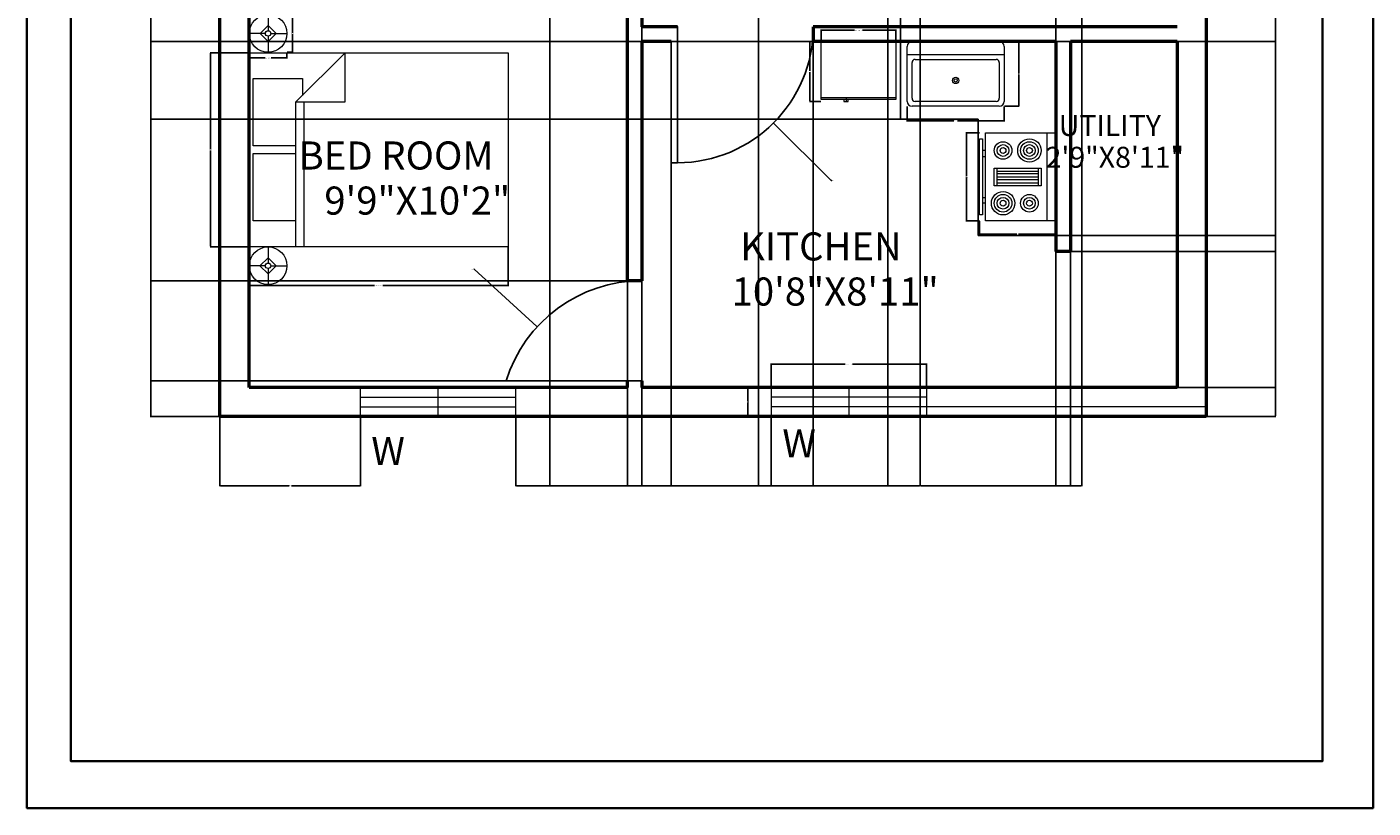
# Model space of a CAD drawing. Units: inches. Extents: x 1804 to 2221, y 1838 to 2403.
# Tile 1 of 3: x 1804 to 2221, y 1838 to 2079. Entities that reach past the tile are written whole.
import ezdxf

# ---------------------------------------------------------------- set-up
doc = ezdxf.new("R2010")
doc.units = ezdxf.units.IN
for name, color, linetype, lineweight in [('A-ANNO-DIMS', 2, 'Continuous', 18), ('A-ANNO-TEXT', 7, 'Continuous', 25), ('A-ANNO-TTLB', 7, 'Continuous', 35), ('A-AREA-IDEN', 7, 'Continuous', 25), ('A-DOOR', 3, 'Continuous', 25), ('A-EQPM', 8, 'Continuous', 18), ('A-FLOR-CASE', 8, 'Continuous', 25), ('A-FLOR-FIXT', 9, 'Continuous', 18), ('A-FURN', 8, 'Continuous', 18), ('A-GLAZ', 4, 'Continuous', 18), ('A-WALL', 7, 'Continuous', 50)]:
    doc.layers.add(name, color=color, linetype=linetype, lineweight=lineweight)
doc.styles.get("Standard").update_dxf_attribs({"font": 'arial.ttf'})
doc.dimstyles.get("Standard").update_dxf_attribs({"dimtxt": 0.18, "dimasz": 0.18, "dimexe": 0.18, "dimexo": 0.0625, "dimgap": 0.09, "dimtad": 0, "dimtih": 1, "dimtoh": 1, "dimdec": 4, "dimzin": 0, "dimdsep": 46, "dimtxsty": 'Standard', "dimcen": 0.09, "dimadec": 0, "dimazin": 0, "dimtfac": 1, "dimtdec": 4, "dimtofl": 0, "dimtmove": 0, "dimatfit": 3, "dimfxl": 1, "dimtolj": 1, "dimtzin": 0, "dimarcsym": 0})

# ---------------------------------------------------------------- blocks, each defined once
blk = doc.blocks.new('Range-Oven - 30 in top')
for p, q in [((0, -3), (30, -3)), ((12, -6), (18, -6)), ((13, -20), (13, -6)), ((14, -6), (14, -20)), ((15, -20), (15, -6)), ((16, -6), (16, -20)), ((17, -20), (17, -6)), ((18, -20), (12, -20)), ((6, -24), (6, -25)), ((8, -25), (8, -24)), ((22, -25), (22, -24)), ((24, -24), (24, -25))]:
    blk.add_line(p, q)
for points in [[(0, -24), (0, 0), (30, 0), (30, -24)], [(12, -21), (12, -5), (18, -5), (18, -21)], [(2, -26), (2, -25), (28, -25), (28, -26)]]:
    blk.add_lwpolyline(points, close=True)
for centre, radius in [((6, -9), 4), ((6, -9), 3), ((6, -9), 2), ((6, -9), 1), ((24, -9), 3), ((24, -9), 2), ((24, -9), 1), ((6, -18), 3), ((6, -18), 2), ((6, -18), 1), ((24, -18), 4), ((24, -18), 3), ((24, -18), 2), ((24, -18), 1)]:
    blk.add_circle(centre, radius)
blk = doc.blocks.new('Bed - Queen')
for p, q in [((0, -80.00003), (0, 0)), ((0, 0), (59.99999, 0)), ((59.99999, 0), (59.99999, -80.00003)), ((7.99999, -1.2), (28.79998, -1.2)), ((7.99999, -14.4), (7.99999, -1.2)), ((28.79998, -1.2), (28.79998, -14.4)), ((31.19999, -1.2), (51.99999, -1.2)), ((31.19999, -14.4), (31.19999, -1.2)), ((51.99999, -1.2), (51.99999, -16.4)), ((0, -14.4), (44.8, -14.4)), ((59.99999, -29.6), (44.8, -14.4)), ((44.8, -14.4), (44.8, -29.6)), ((51.99999, -16.4), (46.79936, -16.4)), ((44.8, -16.8), (0, -16.8)), ((44.8, -29.6), (59.99999, -29.6)), ((59.99999, -80.00003), (0, -80.00003))]:
    blk.add_line(p, q)
blk = doc.blocks.new('Lamp - Table')
for p, q in [((0, 7), (0, 1)), ((-1, 0), (-7, 0)), ((0, 3), (-3, 0)), ((-3, 0), (0, -3)), ((3, 0), (0, 3)), ((0, -3), (3, 0)), ((1, 0), (7, 0)), ((0, -1), (0, -7))]:
    blk.add_line(p, q)
for radius in [7, 1]:
    blk.add_circle((0, 0), radius)
blk = doc.blocks.new('Refrigerator-2 door - 36 in top')
for p, q in [((0, -26.999999), (36, -26.999999)), ((11, -27.999999), (11, -28.999999)), ((11, -28.999999), (13, -28.999999)), ((12, -26.999999), (12, -28.999999)), ((13, -28.999999), (13, -27.999999))]:
    blk.add_line(p, q)
blk.add_lwpolyline([(0, -27.999999), (0, 0), (36, 0), (36, -27.999999)], close=True)
blk = doc.blocks.new('Sink-single - 30 in top')
blk.add_line((-15, -3.999996), (15, -3.999996))
for points in [[(-13.5, 0), (13.5, 0)], [(-15, -18.499996), (-15, -1.5)], [(15, -1.5), (15, -18.499996)], [(-13.5, -17.499996), (-13.5, -6.499996)], [(-12.5, -5.499996), (12.5, -5.499996)], [(13.5, -6.499996), (13.5, -17.499996)], [(13.5, -19.999996), (-13.5, -19.999996)], [(12.5, -18.499996), (-12.5, -18.499996)]]:
    blk.add_lwpolyline(points)
for radius in [1, 0.5]:
    blk.add_circle((0, -11.999996), radius)
for centre, radius, start, end in [((-13.5, -1.5), 1.5, 90, 180), ((13.5, -1.5), 1.5, 0, 90), ((-12.5, -6.499996), 1, 90, 180), ((12.5, -6.499996), 1, 0, 90), ((-13.5, -18.499996), 1.5, 180, 270), ((-12.5, -17.499996), 1, 180, 270), ((12.5, -17.499996), 1, 270, 0), ((13.5, -18.499996), 1.5, 270, 0)]:
    blk.add_arc(centre, radius, start, end)
blk = doc.blocks.new('WIN-48IN-DOUBLE-PANEL')
for p, q in [((0, 9), (0, 0)), ((24, 9), (24, 0)), ((48, 9), (48, 0)), ((48, 6), (0, 6)), ((48, 3), (0, 3))]:
    blk.add_line(p, q)
blk = doc.blocks.new('*D12')
at = {"layer": 'A-ANNO-DIMS', "color": 0, "lineweight": -2, "transparency": 16777216}
for p, q in [((1873.17, 2071.56), (1873.17, 2069.7)), ((1873.35, 2069.88), (1878.1, 2069.88)), ((1884.64, 2069.88), (1879.9, 2069.88)), ((1884.82, 2071.56), (1884.82, 2069.7))]:
    blk.add_line(p, q, dxfattribs=at)
at = {"layer": 'A-ANNO-DIMS', "color": 0, "transparency": 16777216}
for points in [[(1873.35, 2069.91), (1873.35, 2069.85), (1873.17, 2069.88)], [(1884.64, 2069.91), (1884.64, 2069.85), (1884.82, 2069.88)]]:
    blk.add_solid(points, dxfattribs=at)
at = {"layer": 'Defpoints', "color": 0, "transparency": 16777216}
for p in [(1873.17, 2071.62), (1884.82, 2071.62), (1884.82, 2069.88)]:
    blk.add_point(p, dxfattribs=at)
at = {"layer": 'A-ANNO-DIMS', "color": 0, "transparency": 16777216, "insert": (1879, 2069.88), "char_height": 0.18, "attachment_point": 5}
blk.add_mtext('\\A1;LAMP 12 TYP.', dxfattribs=at)
blk = doc.blocks.new('*D13')
at = {"layer": 'A-ANNO-DIMS', "color": 0, "lineweight": -2, "transparency": 16777216}
for p, q in [((1884.89, 2083.28), (1886.75, 2083.28)), ((1886.57, 2083.1), (1886.57, 2077.63)), ((1886.57, 2071.8), (1886.57, 2077.27)), ((1884.89, 2071.62), (1886.75, 2071.62))]:
    blk.add_line(p, q, dxfattribs=at)
at = {"layer": 'A-ANNO-DIMS', "color": 0, "transparency": 16777216}
for points in [[(1886.54, 2083.1), (1886.6, 2083.1), (1886.57, 2083.28)], [(1886.54, 2071.8), (1886.6, 2071.8), (1886.57, 2071.62)]]:
    blk.add_solid(points, dxfattribs=at)
at = {"layer": 'Defpoints', "color": 0, "transparency": 16777216}
for p in [(1884.82, 2083.28), (1886.57, 2083.28), (1884.82, 2071.62)]:
    blk.add_point(p, dxfattribs=at)
at = {"layer": 'A-ANNO-DIMS', "color": 0, "transparency": 16777216, "insert": (1886.57, 2077.45), "char_height": 0.18, "attachment_point": 5}
blk.add_mtext('\\A1;12 TYP.', dxfattribs=at)
blk = doc.blocks.new('*D14')
at = {"layer": 'A-ANNO-DIMS', "color": 0, "lineweight": -2, "transparency": 16777216}
for p, q in [((1873.21, 2011.42), (1873.21, 1999.31)), ((1953.21, 2011.42), (1953.21, 1999.31)), ((1873.39, 1999.49), (1911.91, 1999.49)), ((1953.03, 1999.49), (1914.52, 1999.49))]:
    blk.add_line(p, q, dxfattribs=at)
at = {"layer": 'A-ANNO-DIMS', "color": 0, "transparency": 16777216}
for points in [[(1873.39, 1999.52), (1873.39, 1999.46), (1873.21, 1999.49)], [(1953.03, 1999.52), (1953.03, 1999.46), (1953.21, 1999.49)]]:
    blk.add_solid(points, dxfattribs=at)
at = {"layer": 'Defpoints', "color": 0, "transparency": 16777216}
for p in [(1873.21, 2011.49), (1953.21, 2011.49), (1873.21, 1999.49)]:
    blk.add_point(p, dxfattribs=at)
at = {"layer": 'A-ANNO-DIMS', "color": 0, "transparency": 16777216, "insert": (1913.21, 1999.49), "char_height": 0.18, "attachment_point": 5}
blk.add_mtext('\\A1;QUEEN BED 80 TYP.', dxfattribs=at)
blk = doc.blocks.new('*D15')
at = {"layer": 'A-ANNO-DIMS', "color": 0, "lineweight": -2, "transparency": 16777216}
for p, q in [((1873.15, 2071.49), (1861.03, 2071.49)), ((1861.21, 2071.31), (1861.21, 2041.67)), ((1861.21, 2011.67), (1861.21, 2041.3)), ((1873.15, 2011.49), (1861.03, 2011.49))]:
    blk.add_line(p, q, dxfattribs=at)
at = {"layer": 'A-ANNO-DIMS', "color": 0, "transparency": 16777216}
for points in [[(1861.18, 2071.31), (1861.24, 2071.31), (1861.21, 2071.49)], [(1861.18, 2011.67), (1861.24, 2011.67), (1861.21, 2011.49)]]:
    blk.add_solid(points, dxfattribs=at)
at = {"layer": 'Defpoints', "color": 0, "transparency": 16777216}
for p in [(1861.21, 2071.49), (1873.21, 2071.49), (1873.21, 2011.49)]:
    blk.add_point(p, dxfattribs=at)
at = {"layer": 'A-ANNO-DIMS', "color": 0, "transparency": 16777216, "insert": (1861.21, 2041.49), "char_height": 0.18, "attachment_point": 5}
blk.add_mtext('\\A1;60 TYP.', dxfattribs=at)
blk = doc.blocks.new('*D16')
at = {"layer": 'A-ANNO-DIMS', "color": 0, "lineweight": -2, "transparency": 16777216}
for p, q in [((2034.6, 1968.03), (2034.6, 1975.35)), ((2034.78, 1975.17), (2057.48, 1975.17)), ((2082.42, 1975.17), (2059.72, 1975.17)), ((2082.6, 1968.03), (2082.6, 1975.35))]:
    blk.add_line(p, q, dxfattribs=at)
at = {"layer": 'A-ANNO-DIMS', "color": 0, "transparency": 16777216}
for points in [[(2034.78, 1975.2), (2034.78, 1975.14), (2034.6, 1975.17)], [(2082.42, 1975.2), (2082.42, 1975.14), (2082.6, 1975.17)]]:
    blk.add_solid(points, dxfattribs=at)
at = {"layer": 'Defpoints', "color": 0, "transparency": 16777216}
for p in [(2082.6, 1975.17), (2034.6, 1967.97), (2082.6, 1967.97)]:
    blk.add_point(p, dxfattribs=at)
at = {"layer": 'A-ANNO-DIMS', "color": 0, "transparency": 16777216, "insert": (2058.6, 1975.17), "char_height": 0.18, "attachment_point": 5}
blk.add_mtext('\\A1;WINDOW 48 TYP.', dxfattribs=at)
blk = doc.blocks.new('*D17')
at = {"layer": 'A-ANNO-DIMS', "color": 0, "lineweight": -2, "transparency": 16777216}
for p, q in [((2034.54, 1967.97), (2027.22, 1967.97)), ((2027.4, 1967.79), (2027.4, 1963.65)), ((2027.4, 1959.15), (2027.4, 1963.29)), ((2034.54, 1958.97), (2027.22, 1958.97))]:
    blk.add_line(p, q, dxfattribs=at)
at = {"layer": 'A-ANNO-DIMS', "color": 0, "transparency": 16777216}
for points in [[(2027.37, 1967.79), (2027.43, 1967.79), (2027.4, 1967.97)], [(2027.37, 1959.15), (2027.43, 1959.15), (2027.4, 1958.97)]]:
    blk.add_solid(points, dxfattribs=at)
at = {"layer": 'Defpoints', "color": 0, "transparency": 16777216}
for p in [(2027.4, 1967.97), (2034.6, 1967.97), (2034.6, 1958.97)]:
    blk.add_point(p, dxfattribs=at)
at = {"layer": 'A-ANNO-DIMS', "color": 0, "transparency": 16777216, "insert": (2027.4, 1963.47), "char_height": 0.18, "attachment_point": 5}
blk.add_mtext('\\A1;9 TYP.', dxfattribs=at)
blk = doc.blocks.new('*D24')
at = {"layer": 'A-ANNO-DIMS', "color": 0, "lineweight": -2, "transparency": 16777216}
for p, q in [((2098.97, 2046.68), (2094.78, 2046.68)), ((2094.96, 2046.5), (2094.96, 2033.27)), ((2094.96, 2019.68), (2094.96, 2032.91)), ((2098.97, 2019.5), (2094.78, 2019.5))]:
    blk.add_line(p, q, dxfattribs=at)
at = {"layer": 'A-ANNO-DIMS', "color": 0, "transparency": 16777216}
for points in [[(2094.93, 2046.5), (2094.99, 2046.5), (2094.96, 2046.68)], [(2094.93, 2019.68), (2094.99, 2019.68), (2094.96, 2019.5)]]:
    blk.add_solid(points, dxfattribs=at)
at = {"layer": 'Defpoints', "color": 0, "transparency": 16777216}
for p in [(2099.03, 2046.68), (2094.96, 2019.5), (2099.03, 2019.5)]:
    blk.add_point(p, dxfattribs=at)
at = {"layer": 'A-ANNO-DIMS', "color": 0, "transparency": 16777216, "insert": (2094.96, 2033.09), "char_height": 0.18, "attachment_point": 5}
blk.add_mtext('\\A1;RANGE 27', dxfattribs=at)
blk = doc.blocks.new('*D25')
at = {"layer": 'A-ANNO-DIMS', "color": 0, "lineweight": -2, "transparency": 16777216}
for p, q in [((2099.03, 2019.44), (2099.03, 2015.24)), ((2122.59, 2019.44), (2122.59, 2015.24)), ((2099.21, 2015.42), (2110.59, 2015.42)), ((2122.41, 2015.42), (2111.03, 2015.42))]:
    blk.add_line(p, q, dxfattribs=at)
at = {"layer": 'A-ANNO-DIMS', "color": 0, "transparency": 16777216}
for points in [[(2099.21, 2015.45), (2099.21, 2015.39), (2099.03, 2015.42)], [(2122.41, 2015.45), (2122.41, 2015.39), (2122.59, 2015.42)]]:
    blk.add_solid(points, dxfattribs=at)
at = {"layer": 'Defpoints', "color": 0, "transparency": 16777216}
for p in [(2099.03, 2019.5), (2122.59, 2019.5), (2122.59, 2015.42)]:
    blk.add_point(p, dxfattribs=at)
at = {"layer": 'A-ANNO-DIMS', "color": 0, "transparency": 16777216, "insert": (2110.81, 2015.42), "char_height": 0.18, "attachment_point": 5}
blk.add_mtext('\\A1;24', dxfattribs=at)
blk = doc.blocks.new('*D26')
at = {"layer": 'A-ANNO-DIMS', "color": 0, "lineweight": -2, "transparency": 16777216}
for p, q in [((2050.02, 2075.05), (2050.02, 2078.63)), ((2050.2, 2078.45), (2060.32, 2078.45)), ((2072.93, 2078.45), (2062.82, 2078.45)), ((2073.11, 2075.05), (2073.11, 2078.63))]:
    blk.add_line(p, q, dxfattribs=at)
at = {"layer": 'A-ANNO-DIMS', "color": 0, "transparency": 16777216}
for points in [[(2050.2, 2078.48), (2050.2, 2078.42), (2050.02, 2078.45)], [(2072.93, 2078.48), (2072.93, 2078.42), (2073.11, 2078.45)]]:
    blk.add_solid(points, dxfattribs=at)
at = {"layer": 'Defpoints', "color": 0, "transparency": 16777216}
for p in [(2073.11, 2078.45), (2050.02, 2074.99), (2073.11, 2074.99)]:
    blk.add_point(p, dxfattribs=at)
at = {"layer": 'A-ANNO-DIMS', "color": 0, "transparency": 16777216, "insert": (2061.57, 2078.45), "char_height": 0.18, "attachment_point": 5}
blk.add_mtext('\\A1;REFRIGERATOR 23', dxfattribs=at)
blk = doc.blocks.new('*D27')
at = {"layer": 'A-ANNO-DIMS', "color": 0, "lineweight": -2, "transparency": 16777216}
for p, q in [((2049.96, 2074.99), (2046.38, 2074.99)), ((2046.56, 2074.81), (2046.56, 2065.87)), ((2046.56, 2056.57), (2046.56, 2065.51)), ((2049.96, 2056.39), (2046.38, 2056.39))]:
    blk.add_line(p, q, dxfattribs=at)
at = {"layer": 'A-ANNO-DIMS', "color": 0, "transparency": 16777216}
for points in [[(2046.53, 2074.81), (2046.59, 2074.81), (2046.56, 2074.99)], [(2046.53, 2056.57), (2046.59, 2056.57), (2046.56, 2056.39)]]:
    blk.add_solid(points, dxfattribs=at)
at = {"layer": 'Defpoints', "color": 0, "transparency": 16777216}
for p in [(2046.56, 2074.99), (2050.02, 2074.99), (2050.02, 2056.39)]:
    blk.add_point(p, dxfattribs=at)
at = {"layer": 'A-ANNO-DIMS', "color": 0, "transparency": 16777216, "insert": (2046.56, 2065.69), "char_height": 0.18, "attachment_point": 5}
blk.add_mtext('\\A1;19', dxfattribs=at)
blk = doc.blocks.new('*D30')
at = {"layer": 'A-ANNO-DIMS', "color": 0, "lineweight": -2, "transparency": 16777216}
for p, q in [((2076.63, 2054.86), (2076.63, 2050.25)), ((2106.63, 2054.86), (2106.63, 2050.25)), ((2076.81, 2050.43), (2091.08, 2050.43)), ((2106.45, 2050.43), (2092.17, 2050.43))]:
    blk.add_line(p, q, dxfattribs=at)
at = {"layer": 'A-ANNO-DIMS', "color": 0, "transparency": 16777216}
for points in [[(2076.81, 2050.46), (2076.81, 2050.4), (2076.63, 2050.43)], [(2106.45, 2050.46), (2106.45, 2050.4), (2106.63, 2050.43)]]:
    blk.add_solid(points, dxfattribs=at)
at = {"layer": 'Defpoints', "color": 0, "transparency": 16777216}
for p in [(2076.63, 2054.93), (2106.63, 2054.93), (2106.63, 2050.43)]:
    blk.add_point(p, dxfattribs=at)
at = {"layer": 'A-ANNO-DIMS', "color": 0, "transparency": 16777216, "insert": (2091.63, 2050.43), "char_height": 0.18, "attachment_point": 5}
blk.add_mtext('\\A1;SINK 30', dxfattribs=at)
blk = doc.blocks.new('*D31')
at = {"layer": 'A-ANNO-DIMS', "color": 0, "lineweight": -2, "transparency": 16777216}
for p, q in [((2106.69, 2074.93), (2111.31, 2074.93)), ((2111.13, 2074.75), (2111.13, 2065.11)), ((2111.13, 2055.11), (2111.13, 2064.74)), ((2106.69, 2054.93), (2111.31, 2054.93))]:
    blk.add_line(p, q, dxfattribs=at)
at = {"layer": 'A-ANNO-DIMS', "color": 0, "transparency": 16777216}
for points in [[(2111.1, 2074.75), (2111.16, 2074.75), (2111.13, 2074.93)], [(2111.1, 2055.11), (2111.16, 2055.11), (2111.13, 2054.93)]]:
    blk.add_solid(points, dxfattribs=at)
at = {"layer": 'Defpoints', "color": 0, "transparency": 16777216}
for p in [(2106.63, 2074.93), (2111.13, 2074.93), (2106.63, 2054.93)]:
    blk.add_point(p, dxfattribs=at)
at = {"layer": 'A-ANNO-DIMS', "color": 0, "transparency": 16777216, "insert": (2111.13, 2064.93), "char_height": 0.18, "attachment_point": 5}
blk.add_mtext('\\A1;20', dxfattribs=at)
blk = doc.blocks.new('*D33')
at = {"layer": 'A-ANNO-DIMS', "color": 0, "lineweight": -2, "transparency": 16777216}
for p, q in [((1864.04, 2287.97), (1842.52, 2287.97)), ((1842.7, 2287.79), (1842.7, 2123.65)), ((1842.7, 1959.15), (1842.7, 2123.29)), ((1864.04, 1958.97), (1842.52, 1958.97))]:
    blk.add_line(p, q, dxfattribs=at)
at = {"layer": 'A-ANNO-DIMS', "color": 0, "transparency": 16777216}
for points in [[(1842.67, 2287.79), (1842.73, 2287.79), (1842.7, 2287.97)], [(1842.67, 1959.15), (1842.73, 1959.15), (1842.7, 1958.97)]]:
    blk.add_solid(points, dxfattribs=at)
at = {"layer": 'Defpoints', "color": 0, "transparency": 16777216}
for p in [(1842.7, 2287.97), (1864.1, 2287.97), (1864.1, 1958.97)]:
    blk.add_point(p, dxfattribs=at)
at = {"layer": 'A-ANNO-DIMS', "color": 0, "transparency": 16777216, "insert": (1842.7, 2123.47), "char_height": 0.18, "attachment_point": 5}
blk.add_mtext('\\A1;329', dxfattribs=at)
blk = doc.blocks.new('*D35')
at = {"layer": 'A-ANNO-DIMS', "color": 0, "lineweight": -2, "transparency": 16777216}
for p, q in [((1864.1, 1958.91), (1864.1, 1937.39)), ((1907.6, 1958.91), (1907.6, 1937.39)), ((1864.28, 1937.57), (1885.52, 1937.57)), ((1907.42, 1937.57), (1886.18, 1937.57))]:
    blk.add_line(p, q, dxfattribs=at)
at = {"layer": 'A-ANNO-DIMS', "color": 0, "transparency": 16777216}
for points in [[(1864.28, 1937.6), (1864.28, 1937.54), (1864.1, 1937.57)], [(1907.42, 1937.6), (1907.42, 1937.54), (1907.6, 1937.57)]]:
    blk.add_solid(points, dxfattribs=at)
at = {"layer": 'Defpoints', "color": 0, "transparency": 16777216}
for p in [(1864.1, 1958.97), (1907.6, 1958.97), (1907.6, 1937.57)]:
    blk.add_point(p, dxfattribs=at)
at = {"layer": 'A-ANNO-DIMS', "color": 0, "transparency": 16777216, "insert": (1885.85, 1937.57), "char_height": 0.18, "attachment_point": 5}
blk.add_mtext('\\A1;43.5', dxfattribs=at)
blk = doc.blocks.new('*D36')
at = {"layer": 'A-ANNO-DIMS', "color": 0, "lineweight": -2, "transparency": 16777216}
for p, q in [((1955.6, 1958.91), (1955.6, 1937.39)), ((2034.6, 1958.91), (2034.6, 1937.39)), ((1955.78, 1937.57), (1994.88, 1937.57)), ((2034.42, 1937.57), (1995.32, 1937.57))]:
    blk.add_line(p, q, dxfattribs=at)
at = {"layer": 'A-ANNO-DIMS', "color": 0, "transparency": 16777216}
for points in [[(1955.78, 1937.6), (1955.78, 1937.54), (1955.6, 1937.57)], [(2034.42, 1937.6), (2034.42, 1937.54), (2034.6, 1937.57)]]:
    blk.add_solid(points, dxfattribs=at)
at = {"layer": 'Defpoints', "color": 0, "transparency": 16777216}
for p in [(1955.6, 1958.97), (2034.6, 1958.97), (2034.6, 1937.57)]:
    blk.add_point(p, dxfattribs=at)
at = {"layer": 'A-ANNO-DIMS', "color": 0, "transparency": 16777216, "insert": (1995.1, 1937.57), "char_height": 0.18, "attachment_point": 5}
blk.add_mtext('\\A1;79', dxfattribs=at)
blk = doc.blocks.new('*D37')
at = {"layer": 'A-ANNO-DIMS', "color": 0, "lineweight": -2, "transparency": 16777216}
for p, q in [((2169.16, 2093.67), (2190.68, 2093.67)), ((2190.5, 2093.49), (2190.5, 2026.5)), ((2190.5, 1959.15), (2190.5, 2026.14)), ((2169.16, 1958.97), (2190.68, 1958.97))]:
    blk.add_line(p, q, dxfattribs=at)
at = {"layer": 'A-ANNO-DIMS', "color": 0, "transparency": 16777216}
for points in [[(2190.47, 2093.49), (2190.53, 2093.49), (2190.5, 2093.67)], [(2190.47, 1959.15), (2190.53, 1959.15), (2190.5, 1958.97)]]:
    blk.add_solid(points, dxfattribs=at)
at = {"layer": 'Defpoints', "color": 0, "transparency": 16777216}
for p in [(2169.1, 2093.67), (2190.5, 2093.67), (2169.1, 1958.97)]:
    blk.add_point(p, dxfattribs=at)
at = {"layer": 'A-ANNO-DIMS', "color": 0, "transparency": 16777216, "insert": (2190.5, 2026.32), "char_height": 0.18, "attachment_point": 5}
blk.add_mtext('\\A1;134.7', dxfattribs=at)
blk = doc.blocks.new('*D41')
at = {"layer": 'A-ANNO-DIMS', "color": 0, "lineweight": -2, "transparency": 16777216}
for p, q in [((1994.6, 2204.41), (1994.6, 1937.39)), ((2030.6, 2204.41), (2030.6, 1937.39)), ((1994.78, 1937.57), (2012.38, 1937.57)), ((2030.42, 1937.57), (2012.82, 1937.57))]:
    blk.add_line(p, q, dxfattribs=at)
at = {"layer": 'A-ANNO-DIMS', "color": 0, "transparency": 16777216}
for points in [[(1994.78, 1937.6), (1994.78, 1937.54), (1994.6, 1937.57)], [(2030.42, 1937.6), (2030.42, 1937.54), (2030.6, 1937.57)]]:
    blk.add_solid(points, dxfattribs=at)
at = {"layer": 'Defpoints', "color": 0, "transparency": 16777216}
for p in [(1994.6, 2204.47), (2030.6, 2204.47), (2030.6, 1937.57)]:
    blk.add_point(p, dxfattribs=at)
at = {"layer": 'A-ANNO-DIMS', "color": 0, "transparency": 16777216, "insert": (2012.6, 1937.57), "char_height": 0.18, "attachment_point": 5}
blk.add_mtext('\\A1;36', dxfattribs=at)
blk = doc.blocks.new('*D42')
at = {"layer": 'A-ANNO-DIMS', "color": 0, "lineweight": -2, "transparency": 16777216}
for p, q in [((2030.6, 2254.91), (2030.6, 1937.39)), ((2130.6, 2254.91), (2130.6, 1937.39)), ((2030.78, 1937.57), (2080.32, 1937.57)), ((2130.42, 1937.57), (2080.88, 1937.57))]:
    blk.add_line(p, q, dxfattribs=at)
at = {"layer": 'A-ANNO-DIMS', "color": 0, "transparency": 16777216}
for points in [[(2030.78, 1937.6), (2030.78, 1937.54), (2030.6, 1937.57)], [(2130.42, 1937.6), (2130.42, 1937.54), (2130.6, 1937.57)]]:
    blk.add_solid(points, dxfattribs=at)
at = {"layer": 'Defpoints', "color": 0, "transparency": 16777216}
for p in [(2030.6, 2254.97), (2130.6, 2254.97), (2130.6, 1937.57)]:
    blk.add_point(p, dxfattribs=at)
at = {"layer": 'A-ANNO-DIMS', "color": 0, "transparency": 16777216, "insert": (2080.6, 1937.57), "char_height": 0.18, "attachment_point": 5}
blk.add_mtext('\\A1;100', dxfattribs=at)
blk = doc.blocks.new('*D44')
at = {"layer": 'A-ANNO-DIMS', "color": 0, "lineweight": -2, "transparency": 16777216}
for p, q in [((2070.6, 2204.41), (2070.6, 1937.39)), ((2080.6, 2204.41), (2080.6, 1937.39)), ((2070.78, 1937.57), (2075.39, 1937.57)), ((2080.42, 1937.57), (2075.81, 1937.57))]:
    blk.add_line(p, q, dxfattribs=at)
at = {"layer": 'A-ANNO-DIMS', "color": 0, "transparency": 16777216}
for points in [[(2070.78, 1937.6), (2070.78, 1937.54), (2070.6, 1937.57)], [(2080.42, 1937.6), (2080.42, 1937.54), (2080.6, 1937.57)]]:
    blk.add_solid(points, dxfattribs=at)
at = {"layer": 'Defpoints', "color": 0, "transparency": 16777216}
for p in [(2070.6, 2204.47), (2080.6, 2204.47), (2080.6, 1937.57)]:
    blk.add_point(p, dxfattribs=at)
at = {"layer": 'A-ANNO-DIMS', "color": 0, "transparency": 16777216, "insert": (2075.6, 1937.57), "char_height": 0.18, "attachment_point": 5}
blk.add_mtext('\\A1;10', dxfattribs=at)
blk = doc.blocks.new('*D50')
at = {"layer": 'A-ANNO-DIMS', "color": 0, "lineweight": -2, "transparency": 16777216}
for p, q in [((1990.04, 2000.97), (1842.52, 2000.97)), ((1842.7, 2000.79), (1842.7, 1985.65)), ((1842.7, 1970.15), (1842.7, 1985.29)), ((1990.04, 1969.97), (1842.52, 1969.97))]:
    blk.add_line(p, q, dxfattribs=at)
at = {"layer": 'A-ANNO-DIMS', "color": 0, "transparency": 16777216}
for points in [[(1842.67, 2000.79), (1842.73, 2000.79), (1842.7, 2000.97)], [(1842.67, 1970.15), (1842.73, 1970.15), (1842.7, 1969.97)]]:
    blk.add_solid(points, dxfattribs=at)
at = {"layer": 'Defpoints', "color": 0, "transparency": 16777216}
for p in [(1842.7, 2000.97), (1990.1, 2000.97), (1990.1, 1969.97)]:
    blk.add_point(p, dxfattribs=at)
at = {"layer": 'A-ANNO-DIMS', "color": 0, "transparency": 16777216, "insert": (1842.7, 1985.47), "char_height": 0.18, "attachment_point": 5}
blk.add_mtext('\\A1;31', dxfattribs=at)
blk = doc.blocks.new('*D53')
at = {"layer": 'A-ANNO-DIMS', "color": 0, "lineweight": -2, "transparency": 16777216}
for p, q in [((2003.6, 2074.91), (2003.6, 1937.39)), ((2047.6, 2074.91), (2047.6, 1937.39)), ((2003.78, 1937.57), (2025.38, 1937.57)), ((2047.42, 1937.57), (2025.82, 1937.57))]:
    blk.add_line(p, q, dxfattribs=at)
at = {"layer": 'A-ANNO-DIMS', "color": 0, "transparency": 16777216}
for points in [[(2003.78, 1937.6), (2003.78, 1937.54), (2003.6, 1937.57)], [(2047.42, 1937.6), (2047.42, 1937.54), (2047.6, 1937.57)]]:
    blk.add_solid(points, dxfattribs=at)
at = {"layer": 'Defpoints', "color": 0, "transparency": 16777216}
for p in [(2003.6, 2074.97), (2047.6, 2074.97), (2047.6, 1937.57)]:
    blk.add_point(p, dxfattribs=at)
at = {"layer": 'A-ANNO-DIMS', "color": 0, "transparency": 16777216, "insert": (2025.6, 1937.57), "char_height": 0.18, "attachment_point": 5}
blk.add_mtext('\\A1;44', dxfattribs=at)
blk = doc.blocks.new('*D54')
at = {"layer": 'A-ANNO-DIMS', "color": 0, "lineweight": -2, "transparency": 16777216}
for p, q in [((2074.6, 2075.03), (2074.6, 2366.45)), ((2074.78, 2366.27), (2098.38, 2366.27)), ((2122.42, 2366.27), (2098.82, 2366.27)), ((2122.6, 2075.03), (2122.6, 2366.45))]:
    blk.add_line(p, q, dxfattribs=at)
at = {"layer": 'A-ANNO-DIMS', "color": 0, "transparency": 16777216}
for points in [[(2074.78, 2366.3), (2074.78, 2366.24), (2074.6, 2366.27)], [(2122.42, 2366.3), (2122.42, 2366.24), (2122.6, 2366.27)]]:
    blk.add_solid(points, dxfattribs=at)
at = {"layer": 'Defpoints', "color": 0, "transparency": 16777216}
for p in [(2122.6, 2366.27), (2074.6, 2074.97), (2122.6, 2074.97)]:
    blk.add_point(p, dxfattribs=at)
at = {"layer": 'A-ANNO-DIMS', "color": 0, "transparency": 16777216, "insert": (2098.6, 2366.27), "char_height": 0.18, "attachment_point": 5}
blk.add_mtext('\\A1;48', dxfattribs=at)
blk = doc.blocks.new('*D55')
at = {"layer": 'A-ANNO-DIMS', "color": 0, "lineweight": -2, "transparency": 16777216}
for p, q in [((2122.66, 2074.97), (2190.68, 2074.97)), ((2190.5, 2074.79), (2190.5, 2045.15)), ((2190.5, 2015.15), (2190.5, 2044.79)), ((2122.66, 2014.97), (2190.68, 2014.97))]:
    blk.add_line(p, q, dxfattribs=at)
at = {"layer": 'A-ANNO-DIMS', "color": 0, "transparency": 16777216}
for points in [[(2190.47, 2074.79), (2190.53, 2074.79), (2190.5, 2074.97)], [(2190.47, 2015.15), (2190.53, 2015.15), (2190.5, 2014.97)]]:
    blk.add_solid(points, dxfattribs=at)
at = {"layer": 'Defpoints', "color": 0, "transparency": 16777216}
for p in [(2122.6, 2074.97), (2190.5, 2074.97), (2122.6, 2014.97)]:
    blk.add_point(p, dxfattribs=at)
at = {"layer": 'A-ANNO-DIMS', "color": 0, "transparency": 16777216, "insert": (2190.5, 2044.97), "char_height": 0.18, "attachment_point": 5}
blk.add_mtext('\\A1;60', dxfattribs=at)
blk = doc.blocks.new('*D56')
at = {"layer": 'A-ANNO-DIMS', "color": 0, "lineweight": -2, "transparency": 16777216}
for p, q in [((2074.54, 2074.97), (1842.52, 2074.97)), ((1842.7, 2074.79), (1842.7, 2063.15)), ((1842.7, 2051.15), (1842.7, 2062.79)), ((2074.54, 2050.97), (1842.52, 2050.97))]:
    blk.add_line(p, q, dxfattribs=at)
at = {"layer": 'A-ANNO-DIMS', "color": 0, "transparency": 16777216}
for points in [[(1842.67, 2074.79), (1842.73, 2074.79), (1842.7, 2074.97)], [(1842.67, 2051.15), (1842.73, 2051.15), (1842.7, 2050.97)]]:
    blk.add_solid(points, dxfattribs=at)
at = {"layer": 'Defpoints', "color": 0, "transparency": 16777216}
for p in [(1842.7, 2074.97), (2074.6, 2074.97), (2074.6, 2050.97)]:
    blk.add_point(p, dxfattribs=at)
at = {"layer": 'A-ANNO-DIMS', "color": 0, "transparency": 16777216, "insert": (1842.7, 2062.97), "char_height": 0.18, "attachment_point": 5}
blk.add_mtext('\\A1;24', dxfattribs=at)
blk = doc.blocks.new('*D57')
at = {"layer": 'A-ANNO-DIMS', "color": 0, "lineweight": -2, "transparency": 16777216}
for p, q in [((2122.6, 2009.91), (2122.6, 1937.39)), ((2127.1, 2009.91), (2127.1, 1937.39)), ((2122.78, 1937.57), (2124.59, 1937.57)), ((2126.92, 1937.57), (2125.11, 1937.57))]:
    blk.add_line(p, q, dxfattribs=at)
at = {"layer": 'A-ANNO-DIMS', "color": 0, "transparency": 16777216}
for points in [[(2122.78, 1937.6), (2122.78, 1937.54), (2122.6, 1937.57)], [(2126.92, 1937.6), (2126.92, 1937.54), (2127.1, 1937.57)]]:
    blk.add_solid(points, dxfattribs=at)
at = {"layer": 'Defpoints', "color": 0, "transparency": 16777216}
for p in [(2122.6, 2009.97), (2127.1, 2009.97), (2127.1, 1937.57)]:
    blk.add_point(p, dxfattribs=at)
at = {"layer": 'A-ANNO-DIMS', "color": 0, "transparency": 16777216, "insert": (2124.85, 1937.57), "char_height": 0.18, "attachment_point": 5}
blk.add_mtext('\\A1;4.5', dxfattribs=at)
blk = doc.blocks.new('*D58')
at = {"layer": 'A-ANNO-DIMS', "color": 0, "lineweight": -2, "transparency": 16777216}
for p, q in [((2127.16, 2009.97), (2190.68, 2009.97)), ((2190.5, 2009.79), (2190.5, 1989.15)), ((2190.5, 1968.15), (2190.5, 1988.79)), ((2122.66, 1967.97), (2190.68, 1967.97))]:
    blk.add_line(p, q, dxfattribs=at)
at = {"layer": 'A-ANNO-DIMS', "color": 0, "transparency": 16777216}
for points in [[(2190.47, 2009.79), (2190.53, 2009.79), (2190.5, 2009.97)], [(2190.47, 1968.15), (2190.53, 1968.15), (2190.5, 1967.97)]]:
    blk.add_solid(points, dxfattribs=at)
at = {"layer": 'Defpoints', "color": 0, "transparency": 16777216}
for p in [(2127.1, 2009.97), (2190.5, 2009.97), (2122.6, 1967.97)]:
    blk.add_point(p, dxfattribs=at)
at = {"layer": 'A-ANNO-DIMS', "color": 0, "transparency": 16777216, "insert": (2190.5, 1988.97), "char_height": 0.18, "attachment_point": 5}
blk.add_mtext('\\A1;42', dxfattribs=at)
blk = doc.blocks.new('*D59')
at = {"layer": 'A-ANNO-DIMS', "color": 0, "lineweight": -2, "transparency": 16777216}
for p, q in [((1966.1, 2154.91), (1966.1, 1937.39)), ((1990.1, 2154.91), (1990.1, 1937.39)), ((1966.28, 1937.57), (1977.88, 1937.57)), ((1989.92, 1937.57), (1978.32, 1937.57))]:
    blk.add_line(p, q, dxfattribs=at)
at = {"layer": 'A-ANNO-DIMS', "color": 0, "transparency": 16777216}
for points in [[(1966.28, 1937.6), (1966.28, 1937.54), (1966.1, 1937.57)], [(1989.92, 1937.6), (1989.92, 1937.54), (1990.1, 1937.57)]]:
    blk.add_solid(points, dxfattribs=at)
at = {"layer": 'Defpoints', "color": 0, "transparency": 16777216}
for p in [(1966.1, 2154.97), (1990.1, 2154.97), (1990.1, 1937.57)]:
    blk.add_point(p, dxfattribs=at)
at = {"layer": 'A-ANNO-DIMS', "color": 0, "transparency": 16777216, "insert": (1978.1, 1937.57), "char_height": 0.18, "attachment_point": 5}
blk.add_mtext('\\A1;24', dxfattribs=at)
blk = doc.blocks.new('*D61')
at = {"layer": 'A-ANNO-DIMS', "color": 0, "lineweight": -2, "transparency": 16777216}
for p, q in [((2005.51, 2079.47), (2005.69, 2079.47)), ((2005.6, 2079.38), (2005.6, 2079.56)), ((2053.12, 2031.95), (2035.43, 2049.64)), ((2053.3, 2031.95), (2053.12, 2031.95))]:
    blk.add_line(p, q, dxfattribs=at)
at = {"layer": 'A-ANNO-DIMS', "color": 0, "transparency": 16777216}
blk.add_solid([(2035.45, 2049.66), (2035.41, 2049.62), (2035.3, 2049.77)], dxfattribs=at)
at = {"layer": 'Defpoints', "color": 0, "transparency": 16777216}
for p in [(2005.6, 2079.47), (2035.3, 2049.77)]:
    blk.add_point(p, dxfattribs=at)
at = {"layer": 'A-ANNO-DIMS', "color": 0, "transparency": 16777216, "insert": (2053.6, 2031.95), "char_height": 0.18, "attachment_point": 5}
blk.add_mtext('\\A1;R42', dxfattribs=at)
blk = doc.blocks.new('*D64')
at = {"layer": 'A-ANNO-DIMS', "color": 0, "lineweight": -2, "transparency": 16777216}
for p, q in [((1942.59, 2004.55), (1942.77, 2004.55)), ((1942.77, 2004.55), (1962.08, 1986.85)), ((1994.51, 1957.02), (1994.69, 1957.02)), ((1994.6, 1956.93), (1994.6, 1957.11))]:
    blk.add_line(p, q, dxfattribs=at)
at = {"layer": 'A-ANNO-DIMS', "color": 0, "transparency": 16777216}
blk.add_solid([(1962.1, 1986.87), (1962.06, 1986.82), (1962.21, 1986.72)], dxfattribs=at)
at = {"layer": 'Defpoints', "color": 0, "transparency": 16777216}
for p in [(1962.21, 1986.72), (1994.6, 1957.02)]:
    blk.add_point(p, dxfattribs=at)
at = {"layer": 'A-ANNO-DIMS', "color": 0, "transparency": 16777216, "insert": (1942.11, 2004.55), "char_height": 0.18, "attachment_point": 5}
blk.add_mtext('\\A1;R43.95', dxfattribs=at)

msp = doc.modelspace()

# ---------------------------------------------------------------- linework, layer by layer
at = {"layer": 'A-ANNO-TTLB'}
for points in [[(1804.4104, 2402.5437), (2220.7086, 2402.5437), (2220.7086, 1837.8762), (1804.4104, 1837.8762)], [(1817.9401, 2390.0649), (2205.0975, 2390.0649), (2205.0975, 1852.4349), (1817.9401, 1852.4349)]]:
    msp.add_lwpolyline(points, close=True, dxfattribs=at)
at = {"layer": 'A-DOOR'}
for p, q in [((2005.6006, 2079.4683), (2005.6006, 2037.4683)), ((2003.6006, 2074.9683), (2003.6006, 2037.4683)), ((2003.6006, 2037.4683), (2005.6006, 2037.4683)), ((1994.6006, 1969.9683), (1952.6006, 1969.9683))]:
    msp.add_line(p, q, dxfattribs=at)
for centre, radius, start, end in [((2005.6006, 2079.4683), 42, 270, 0), ((1994.6006, 1957.0167), 43.9516, 90, 162.861716)]:
    msp.add_arc(centre, radius, start, end, dxfattribs=at)
at = {"layer": 'A-FLOR-CASE'}
for p, q in [((2074.6006, 2074.9683), (2074.6006, 2050.9683)), ((2098.6006, 2050.9683), (2074.6006, 2050.9683)), ((2098.6006, 2050.9683), (2098.6006, 2014.9683)), ((2122.6006, 2014.9683), (2098.6006, 2014.9683))]:
    msp.add_line(p, q, dxfattribs=at)
at = {"layer": 'A-GLAZ'}
msp.add_line((2169.1006, 1961.9683), (2034.6006, 1961.9683), dxfattribs=at)
at = {"layer": 'A-WALL'}
for p, q in [((2169.1006, 2287.9683), (2169.1006, 1958.9683)), ((1864.1006, 1958.9683), (1864.1006, 2278.9683)), ((1994.6006, 2094.4683), (1994.6006, 2079.4683)), ((1873.1006, 1967.9683), (1873.1006, 2089.9683)), ((1990.1006, 2000.9683), (1990.1006, 2089.9683)), ((2005.6006, 2079.4683), (1994.6006, 2079.4683)), ((2160.1006, 2079.4683), (2047.6006, 2079.4683)), ((2047.6006, 2079.4683), (2047.6006, 2074.9683)), ((2003.6006, 2074.9683), (1994.6006, 2074.9683)), ((1994.6006, 2074.9683), (1994.6006, 2000.9683)), ((2122.6006, 2074.9683), (2047.6006, 2074.9683)), ((2122.6006, 2074.9683), (2122.6006, 2009.9683)), ((2127.1006, 2074.9683), (2127.1006, 2009.9683)), ((2160.1006, 2074.9683), (2127.1006, 2074.9683)), ((2160.1006, 2074.9683), (2160.1006, 1967.9683)), ((2127.1006, 2009.9683), (2122.6006, 2009.9683)), ((1994.6006, 2000.9683), (1990.1006, 2000.9683)), ((1990.1006, 1967.9683), (1990.1006, 1969.9683)), ((1994.6006, 1969.9683), (1994.6006, 1967.9683)), ((1990.1006, 1967.9683), (1873.1006, 1967.9683)), ((2122.6006, 1967.9683), (1994.6006, 1967.9683)), ((2160.1006, 1967.9683), (2122.6006, 1967.9683)), ((2169.1006, 1958.9683), (1864.1006, 1958.9683))]:
    msp.add_line(p, q, dxfattribs=at)

# ---------------------------------------------------------------- block references
at = {"layer": 'A-EQPM', "xscale": 0.6414314805435485, "yscale": 0.6414314805435485, "zscale": 0.6414314805435485}
msp.add_blockref('Refrigerator-2 door - 36 in top', (2050.0232, 2074.9896), dxfattribs=at)
at = {"layer": 'A-EQPM', "xscale": 0.9058795288083388, "yscale": 0.9058795288083388, "zscale": 0.9058795288083388, "rotation": 270}
msp.add_blockref('Range-Oven - 30 in top', (2122.5864, 2046.6778), dxfattribs=at)
at = {"layer": 'A-FLOR-FIXT'}
msp.add_blockref('Sink-single - 30 in top', (2091.6265, 2074.9253), dxfattribs=at)
at = {"layer": 'A-FURN', "xscale": 0.8325724254019075, "yscale": 0.8325724254019075, "zscale": 0.8325724254019075}
for p in [(1878.9968, 2077.4528), (1878.9863, 2005.5978)]:
    msp.add_blockref('Lamp - Table', p, dxfattribs=at)
at = {"layer": 'A-FURN', "rotation": 89.99999999999999}
msp.add_blockref('Bed - Queen', (1873.214, 2011.4856), dxfattribs=at)
at = {"layer": 'A-GLAZ', "rotation": 180}
msp.add_blockref('WIN-48IN-DOUBLE-PANEL', (1955.6002, 1967.9686), dxfattribs=at)
at = {"layer": 'A-GLAZ'}
msp.add_blockref('WIN-48IN-DOUBLE-PANEL', (2034.601, 1958.968), dxfattribs=at)

# ---------------------------------------------------------------- texts
at = {"layer": 'A-ANNO-TEXT'}
for p in [(1855.1805, 1943.9826), (1982.2977, 1946.3447)]:
    msp.add_text('                     W', height=8.682741, dxfattribs=at).set_placement(p)
at = {"layer": 'A-AREA-IDEN'}
for s, height, p in [('  UTILITY', 6.47098, (2119.5384, 2045.7416)), ('BED ROOM', 8.68274, (1888.4265, 2035.3616)), ('   2\'9"X8\'11"', 6.470976, (2113.4928, 2035.9219)), ('   9\'9"X10\'2"', 8.682741, (1888.4265, 2021.4135)), ('   KITCHEN', 8.68274, (2017.0261, 2007.2368)), ('  10\'8"X8\'11"', 8.682741, (2017.0261, 1993.2887))]:
    msp.add_text(s, height=height, dxfattribs=at).set_placement(p)

# ---------------------------------------------------------------- dimensions: what is measured, and where the dimension line sits
at = {"layer": 'A-ANNO-DIMS'}
for base, p1, p2, override, picture, middle in [((2122.6006, 2366.2659), (2074.6006, 2074.9683), (2122.6006, 2074.9683), {"dimdec": 0, "dimlfac": 1, "dimrnd": 0, "dimzin": 0, "dimdsep": 46, "dimlunit": 2}, '*D54', (2098.6006, 2366.2659)), ((2130.6006, 1937.5683), (2030.6006, 2254.9683), (2130.6006, 2254.9683), {"dimdec": 0, "dimlfac": 1, "dimrnd": 0, "dimzin": 0, "dimdsep": 46, "dimlunit": 2}, '*D42', (2080.6006, 1937.5683)), ((2030.6006, 1937.5683), (1994.6006, 2204.4683), (2030.6006, 2204.4683), {"dimdec": 0, "dimlfac": 1, "dimrnd": 0, "dimzin": 0, "dimdsep": 46, "dimlunit": 2}, '*D41', (2012.6006, 1937.5683)), ((2080.6006, 1937.5683), (2070.6006, 2204.4683), (2080.6006, 2204.4683), {"dimdec": 0, "dimlfac": 1, "dimrnd": 0, "dimzin": 0, "dimdsep": 46, "dimlunit": 2}, '*D44', (2075.6006, 1937.5683)), ((1990.1006, 1937.5683), (1966.1006, 2154.9683), (1990.1006, 2154.9683), {"dimdec": 0, "dimlfac": 1, "dimrnd": 0, "dimzin": 0, "dimdsep": 46, "dimlunit": 2}, '*D59', (1978.1006, 1937.5683)), ((2047.6006, 1937.5683), (2003.6006, 2074.9683), (2047.6006, 2074.9683), {"dimdec": 0, "dimlfac": 1, "dimrnd": 0, "dimzin": 0, "dimdsep": 46, "dimlunit": 2}, '*D53', (2025.6006, 1937.5683)), ((2122.5864, 2015.425), (2099.0335, 2019.5014), (2122.5864, 2019.5014), {"dimdec": 0, "dimlfac": 1, "dimrnd": 0, "dimzin": 0, "dimdsep": 46, "dimlunit": 2}, '*D25', (2110.81, 2015.425)), ((2127.1006, 1937.5683), (2122.6006, 2009.9683), (2127.1006, 2009.9683), {"dimdec": 1, "dimlfac": 1, "dimrnd": 0, "dimzin": 0, "dimdsep": 46, "dimlunit": 2}, '*D57', (2124.8506, 1937.5683)), ((1907.6006, 1937.5683), (1864.1006, 1958.9683), (1907.6006, 1958.9683), {"dimdec": 1, "dimlfac": 1, "dimrnd": 0, "dimzin": 0, "dimdsep": 46, "dimlunit": 2}, '*D35', (1885.8506, 1937.5683)), ((2034.6006, 1937.5683), (1955.6006, 1958.9683), (2034.6006, 1958.9683), {"dimdec": 0, "dimlfac": 1, "dimrnd": 0, "dimzin": 0, "dimdsep": 46, "dimlunit": 2}, '*D36', (1995.1006, 1937.5683))]:
    dim = msp.add_linear_dim(base=base, p1=p1, p2=p2, dimstyle='Standard', override=override, dxfattribs=at)
    dim.commit()
    dim.dimension.update_dxf_attribs({"geometry": picture, "text_midpoint": middle})
for base, p1, p2, override, picture, middle in [((1842.7006, 2287.9683), (1864.1006, 1958.9683), (1864.1006, 2287.9683), {"dimdec": 0, "dimlfac": 1, "dimrnd": 0, "dimzin": 0, "dimdsep": 46, "dimlunit": 2}, '*D33', (1842.7006, 2123.4683)), ((2190.5006, 2093.6724), (2169.1006, 1958.9683), (2169.1006, 2093.6724), {"dimdec": 1, "dimlfac": 1, "dimrnd": 0, "dimzin": 0, "dimdsep": 46, "dimlunit": 2}, '*D37', (2190.5006, 2026.3204)), ((1842.7006, 2074.9683), (2074.6006, 2050.9683), (2074.6006, 2074.9683), {"dimdec": 0, "dimlfac": 1, "dimrnd": 0, "dimzin": 0, "dimdsep": 46, "dimlunit": 2}, '*D56', (1842.7006, 2062.9683)), ((2046.5594, 2074.9896), (2050.0232, 2056.3881), (2050.0232, 2074.9896), {"dimdec": 0, "dimlfac": 1, "dimrnd": 0, "dimzin": 0, "dimdsep": 46, "dimlunit": 2}, '*D27', (2046.5594, 2065.6889)), ((2111.1265, 2074.9253), (2106.6265, 2054.9253), (2106.6265, 2074.9253), {"dimdec": 0, "dimlfac": 1, "dimrnd": 0, "dimzin": 0, "dimdsep": 46, "dimlunit": 2}, '*D31', (2111.1265, 2064.9253)), ((2190.5006, 2074.9683), (2122.6006, 2014.9683), (2122.6006, 2074.9683), {"dimdec": 0, "dimlfac": 1, "dimrnd": 0, "dimzin": 0, "dimdsep": 46, "dimlunit": 2}, '*D55', (2190.5006, 2044.9683)), ((2190.5006, 2009.9683), (2122.6006, 1967.9683), (2127.1006, 2009.9683), {"dimdec": 0, "dimlfac": 1, "dimrnd": 0, "dimzin": 0, "dimdsep": 46, "dimlunit": 2}, '*D58', (2190.5006, 1988.9683)), ((1842.7006, 2000.9683), (1990.1006, 1969.9683), (1990.1006, 2000.9683), {"dimdec": 0, "dimlfac": 1, "dimrnd": 0, "dimzin": 0, "dimdsep": 46, "dimlunit": 2}, '*D50', (1842.7006, 1985.4683))]:
    dim = msp.add_linear_dim(base=base, p1=p1, p2=p2, angle=90, dimstyle='Standard', override=override, dxfattribs=at)
    dim.commit()
    dim.dimension.update_dxf_attribs({"geometry": picture, "text_midpoint": middle})
for base, p1, p2, angle, text, picture, middle in [((1886.5733, 2083.2808), (1884.8249, 2071.6248), (1884.8249, 2083.2808), 90, '<> TYP.', '*D13', (1886.5733, 2077.4528)), ((1861.214, 2071.4856), (1873.214, 2011.4856), (1873.214, 2071.4856), 90, '<> TYP.', '*D15', (1861.214, 2041.4856)), ((2094.9571, 2019.5014), (2099.0335, 2046.6778), (2099.0335, 2019.5014), 270, 'RANGE <>', '*D24', (2094.9571, 2033.0896)), ((1873.214, 1999.4856), (1953.2141, 2011.4856), (1873.214, 2011.4856), 180, 'QUEEN BED <> TYP.', '*D14', (1913.214, 1999.4856)), ((2027.4006, 1967.9683), (2034.6006, 1958.9683), (2034.6006, 1967.9683), 90, '<> TYP.', '*D17', (2027.4006, 1963.4683))]:
    dim = msp.add_linear_dim(base=base, p1=p1, p2=p2, angle=angle, text=text, dimstyle='Standard', override={"dimdec": 0, "dimlfac": 1, "dimrnd": 0, "dimzin": 0, "dimdsep": 46, "dimlunit": 2}, dxfattribs=at)
    dim.commit()
    dim.dimension.update_dxf_attribs({"geometry": picture, "text_midpoint": middle})
for center, mpoint, override, picture, middle in [((2005.6006, 2079.4683), (2035.2991, 2049.7699), {"dimdec": 0, "dimlfac": 1, "dimrnd": 0, "dimzin": 0, "dimdsep": 46, "dimlunit": 2}, '*D61', (2053.6024, 2031.9508)), ((1994.6006, 1957.0167), (1962.2094, 1986.7245), {"dimdec": 2, "dimlfac": 1, "dimrnd": 0, "dimzin": 0, "dimdsep": 46, "dimlunit": 2}, '*D64', (1942.1142, 2004.5492))]:
    dim = msp.add_radius_dim(center=center, mpoint=mpoint, dimstyle='Standard', override=override, dxfattribs=at)
    dim.commit()
    dim.dimension.update_dxf_attribs({"geometry": picture, "text_midpoint": middle, "dimtype": 164})
for base, p1, p2, text, picture, middle in [((2073.1147, 2078.4534), (2050.0232, 2074.9896), (2073.1147, 2074.9896), 'REFRIGERATOR <>', '*D26', (2061.5689, 2078.4534)), ((1884.8249, 2069.8764), (1873.1688, 2071.6248), (1884.8249, 2071.6248), 'LAMP <> TYP.', '*D12', (1878.9968, 2069.8764)), ((2106.6265, 2050.4253), (2076.6265, 2054.9253), (2106.6265, 2054.9253), 'SINK <>', '*D30', (2091.6265, 2050.4253)), ((2082.6006, 1975.1683), (2034.6006, 1967.9683), (2082.6006, 1967.9683), 'WINDOW <> TYP.', '*D16', (2058.6006, 1975.1683))]:
    dim = msp.add_linear_dim(base=base, p1=p1, p2=p2, text=text, dimstyle='Standard', override={"dimdec": 0, "dimlfac": 1, "dimrnd": 0, "dimzin": 0, "dimdsep": 46, "dimlunit": 2}, dxfattribs=at)
    dim.commit()
    dim.dimension.update_dxf_attribs({"geometry": picture, "text_midpoint": middle})

doc.saveas('drawing.dxf')
